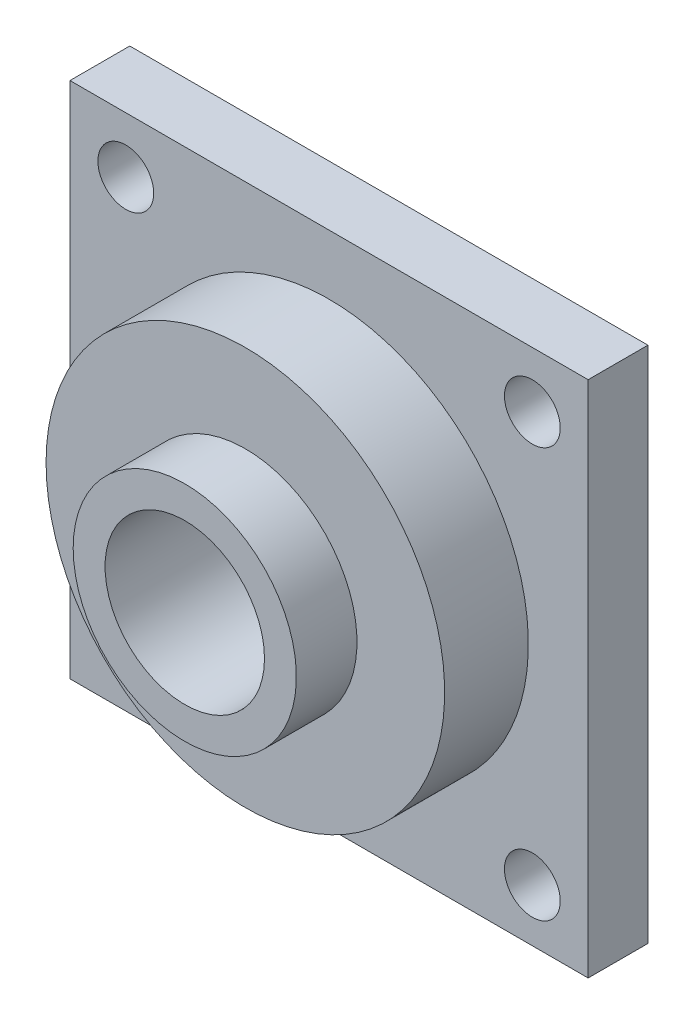
ISO-10303-21;
HEADER;
FILE_DESCRIPTION(('STEP AP214'),'2;1');
FILE_NAME('part.step','',(''),(''),'','','');
FILE_SCHEMA(('AUTOMOTIVE_DESIGN { 1 0 10303 214 1 1 1 1 }'));
ENDSEC;
DATA;
#1=APPLICATION_CONTEXT('core data for automotive mechanical design processes');
#2=APPLICATION_PROTOCOL_DEFINITION('international standard','automotive_design',2000,#1);
#3=PRODUCT_CONTEXT('',#1,'mechanical');
#4=PRODUCT('Part','Part','',(#3));
#5=PRODUCT_RELATED_PRODUCT_CATEGORY('part','',(#4));
#6=PRODUCT_DEFINITION_FORMATION('','',#4);
#7=PRODUCT_DEFINITION_CONTEXT('part definition',#1,'design');
#8=PRODUCT_DEFINITION('design','',#6,#7);
#9=PRODUCT_DEFINITION_SHAPE('','',#8);
#10=(LENGTH_UNIT() NAMED_UNIT(*) SI_UNIT(.MILLI.,.METRE.));
#11=(NAMED_UNIT(*) PLANE_ANGLE_UNIT() SI_UNIT($,.RADIAN.));
#12=(NAMED_UNIT(*) SI_UNIT($,.STERADIAN.) SOLID_ANGLE_UNIT());
#13=UNCERTAINTY_MEASURE_WITH_UNIT(LENGTH_MEASURE(1.E-05),#10,'distance_accuracy_value','');
#14=(GEOMETRIC_REPRESENTATION_CONTEXT(3) GLOBAL_UNCERTAINTY_ASSIGNED_CONTEXT((#13)) GLOBAL_UNIT_ASSIGNED_CONTEXT((#10,
#11,#12)) REPRESENTATION_CONTEXT('',''));
#15=CARTESIAN_POINT('',(0.,0.,0.));
#16=DIRECTION('',(0.,0.,1.));
#17=DIRECTION('',(1.,0.,0.));
#18=AXIS2_PLACEMENT_3D('',#15,#16,#17);
#19=CARTESIAN_POINT('',(0.,130.,15.));
#20=DIRECTION('',(1.,0.,0.));
#21=DIRECTION('',(0.,0.,-1.));
#22=AXIS2_PLACEMENT_3D('',#19,#20,#21);
#23=PLANE('',#22);
#24=DIRECTION('',(0.,-1.,0.));
#25=VECTOR('',#24,1.);
#26=CARTESIAN_POINT('',(0.,130.,0.));
#27=LINE('',#26,#25);
#28=CARTESIAN_POINT('',(0.,130.,0.));
#29=VERTEX_POINT('',#28);
#30=CARTESIAN_POINT('',(0.,0.,0.));
#31=VERTEX_POINT('',#30);
#32=EDGE_CURVE('E115',#29,#31,#27,.T.);
#33=ORIENTED_EDGE('',*,*,#32,.T.);
#34=DIRECTION('',(0.,0.,-1.));
#35=VECTOR('',#34,1.);
#36=CARTESIAN_POINT('',(0.,0.,15.));
#37=LINE('',#36,#35);
#38=CARTESIAN_POINT('',(0.,0.,15.));
#39=VERTEX_POINT('',#38);
#40=EDGE_CURVE('E48',#39,#31,#37,.T.);
#41=ORIENTED_EDGE('',*,*,#40,.F.);
#42=DIRECTION('',(0.,-1.,0.));
#43=VECTOR('',#42,1.);
#44=CARTESIAN_POINT('',(0.,130.,15.));
#45=LINE('',#44,#43);
#46=CARTESIAN_POINT('',(0.,130.,15.));
#47=VERTEX_POINT('',#46);
#48=EDGE_CURVE('E97',#47,#39,#45,.T.);
#49=ORIENTED_EDGE('',*,*,#48,.F.);
#50=DIRECTION('',(0.,0.,-1.));
#51=VECTOR('',#50,1.);
#52=CARTESIAN_POINT('',(0.,130.,15.));
#53=LINE('',#52,#51);
#54=EDGE_CURVE('E107',#47,#29,#53,.T.);
#55=ORIENTED_EDGE('',*,*,#54,.T.);
#56=EDGE_LOOP('',(#33,#41,#49,#55));
#57=FACE_BOUND('',#56,.T.);
#58=ADVANCED_FACE('F44',(#57),#23,.F.);
#59=CARTESIAN_POINT('',(0.,0.,15.));
#60=DIRECTION('',(0.,1.,0.));
#61=DIRECTION('',(0.,0.,1.));
#62=AXIS2_PLACEMENT_3D('',#59,#60,#61);
#63=PLANE('',#62);
#64=DIRECTION('',(1.,0.,0.));
#65=VECTOR('',#64,1.);
#66=CARTESIAN_POINT('',(0.,0.,0.));
#67=LINE('',#66,#65);
#68=CARTESIAN_POINT('',(130.,0.,0.));
#69=VERTEX_POINT('',#68);
#70=EDGE_CURVE('E102',#31,#69,#67,.T.);
#71=ORIENTED_EDGE('',*,*,#70,.T.);
#72=DIRECTION('',(0.,0.,-1.));
#73=VECTOR('',#72,1.);
#74=CARTESIAN_POINT('',(130.,0.,15.));
#75=LINE('',#74,#73);
#76=CARTESIAN_POINT('',(130.,0.,15.));
#77=VERTEX_POINT('',#76);
#78=EDGE_CURVE('E105',#77,#69,#75,.T.);
#79=ORIENTED_EDGE('',*,*,#78,.F.);
#80=DIRECTION('',(1.,0.,0.));
#81=VECTOR('',#80,1.);
#82=CARTESIAN_POINT('',(0.,0.,15.));
#83=LINE('',#82,#81);
#84=EDGE_CURVE('E94',#39,#77,#83,.T.);
#85=ORIENTED_EDGE('',*,*,#84,.F.);
#86=ORIENTED_EDGE('',*,*,#40,.T.);
#87=EDGE_LOOP('',(#71,#79,#85,#86));
#88=FACE_BOUND('',#87,.T.);
#89=ADVANCED_FACE('F103',(#88),#63,.F.);
#90=CARTESIAN_POINT('',(130.,0.,15.));
#91=DIRECTION('',(-1.,0.,0.));
#92=DIRECTION('',(0.,0.,1.));
#93=AXIS2_PLACEMENT_3D('',#90,#91,#92);
#94=PLANE('',#93);
#95=DIRECTION('',(0.,1.,0.));
#96=VECTOR('',#95,1.);
#97=CARTESIAN_POINT('',(130.,0.,0.));
#98=LINE('',#97,#96);
#99=CARTESIAN_POINT('',(130.,130.,0.));
#100=VERTEX_POINT('',#99);
#101=EDGE_CURVE('E76',#69,#100,#98,.T.);
#102=ORIENTED_EDGE('',*,*,#101,.T.);
#103=DIRECTION('',(0.,0.,-1.));
#104=VECTOR('',#103,1.);
#105=CARTESIAN_POINT('',(130.,130.,15.));
#106=LINE('',#105,#104);
#107=CARTESIAN_POINT('',(130.,130.,15.));
#108=VERTEX_POINT('',#107);
#109=EDGE_CURVE('E104',#108,#100,#106,.T.);
#110=ORIENTED_EDGE('',*,*,#109,.F.);
#111=DIRECTION('',(0.,1.,0.));
#112=VECTOR('',#111,1.);
#113=CARTESIAN_POINT('',(130.,0.,15.));
#114=LINE('',#113,#112);
#115=EDGE_CURVE('E100',#77,#108,#114,.T.);
#116=ORIENTED_EDGE('',*,*,#115,.F.);
#117=ORIENTED_EDGE('',*,*,#78,.T.);
#118=EDGE_LOOP('',(#102,#110,#116,#117));
#119=FACE_BOUND('',#118,.T.);
#120=ADVANCED_FACE('F106',(#119),#94,.F.);
#121=CARTESIAN_POINT('',(130.,130.,15.));
#122=DIRECTION('',(0.,-1.,0.));
#123=DIRECTION('',(0.,0.,-1.));
#124=AXIS2_PLACEMENT_3D('',#121,#122,#123);
#125=PLANE('',#124);
#126=DIRECTION('',(-1.,0.,0.));
#127=VECTOR('',#126,1.);
#128=CARTESIAN_POINT('',(130.,130.,0.));
#129=LINE('',#128,#127);
#130=EDGE_CURVE('E88',#100,#29,#129,.T.);
#131=ORIENTED_EDGE('',*,*,#130,.T.);
#132=ORIENTED_EDGE('',*,*,#54,.F.);
#133=DIRECTION('',(-1.,0.,0.));
#134=VECTOR('',#133,1.);
#135=CARTESIAN_POINT('',(130.,130.,15.));
#136=LINE('',#135,#134);
#137=EDGE_CURVE('E63',#108,#47,#136,.T.);
#138=ORIENTED_EDGE('',*,*,#137,.F.);
#139=ORIENTED_EDGE('',*,*,#109,.T.);
#140=EDGE_LOOP('',(#131,#132,#138,#139));
#141=FACE_BOUND('',#140,.T.);
#142=ADVANCED_FACE('F116',(#141),#125,.F.);
#143=CARTESIAN_POINT('',(0.,0.,15.));
#144=DIRECTION('',(0.,0.,1.));
#145=DIRECTION('',(1.,0.,0.));
#146=AXIS2_PLACEMENT_3D('',#143,#144,#145);
#147=PLANE('',#146);
#148=CARTESIAN_POINT('',(116.,13.1965117975312,15.));
#149=DIRECTION('',(0.,0.,1.));
#150=DIRECTION('',(1.,0.,0.));
#151=AXIS2_PLACEMENT_3D('',#148,#149,#150);
#152=CIRCLE('',#151,7.);
#153=CARTESIAN_POINT('',(123.,13.1965117975312,15.));
#154=VERTEX_POINT('',#153);
#155=EDGE_CURVE('E148',#154,#154,#152,.T.);
#156=ORIENTED_EDGE('',*,*,#155,.F.);
#157=EDGE_LOOP('',(#156));
#158=FACE_BOUND('',#157,.T.);
#159=CARTESIAN_POINT('',(14.,14.,15.));
#160=DIRECTION('',(0.,0.,1.));
#161=DIRECTION('',(1.,0.,0.));
#162=AXIS2_PLACEMENT_3D('',#159,#160,#161);
#163=CIRCLE('',#162,7.);
#164=CARTESIAN_POINT('',(21.,14.,15.));
#165=VERTEX_POINT('',#164);
#166=EDGE_CURVE('E155',#165,#165,#163,.T.);
#167=ORIENTED_EDGE('',*,*,#166,.F.);
#168=EDGE_LOOP('',(#167));
#169=FACE_BOUND('',#168,.T.);
#170=CARTESIAN_POINT('',(14.,116.,15.));
#171=DIRECTION('',(0.,0.,1.));
#172=DIRECTION('',(1.,0.,0.));
#173=AXIS2_PLACEMENT_3D('',#170,#171,#172);
#174=CIRCLE('',#173,7.00000000000001);
#175=CARTESIAN_POINT('',(21.,116.,15.));
#176=VERTEX_POINT('',#175);
#177=EDGE_CURVE('E158',#176,#176,#174,.T.);
#178=ORIENTED_EDGE('',*,*,#177,.F.);
#179=EDGE_LOOP('',(#178));
#180=FACE_BOUND('',#179,.T.);
#181=CARTESIAN_POINT('',(116.,116.,15.));
#182=DIRECTION('',(0.,0.,1.));
#183=DIRECTION('',(1.,0.,0.));
#184=AXIS2_PLACEMENT_3D('',#181,#182,#183);
#185=CIRCLE('',#184,7.);
#186=CARTESIAN_POINT('',(123.,116.,15.));
#187=VERTEX_POINT('',#186);
#188=EDGE_CURVE('E137',#187,#187,#185,.T.);
#189=ORIENTED_EDGE('',*,*,#188,.F.);
#190=EDGE_LOOP('',(#189));
#191=FACE_BOUND('',#190,.T.);
#192=CARTESIAN_POINT('',(65.,65.,15.));
#193=DIRECTION('',(0.,0.,1.));
#194=DIRECTION('',(1.,0.,0.));
#195=AXIS2_PLACEMENT_3D('',#192,#193,#194);
#196=CIRCLE('',#195,50.);
#197=CARTESIAN_POINT('',(15.,65.,15.));
#198=VERTEX_POINT('',#197);
#199=EDGE_CURVE('E53',#198,#198,#196,.T.);
#200=ORIENTED_EDGE('',*,*,#199,.F.);
#201=EDGE_LOOP('',(#200));
#202=FACE_BOUND('',#201,.T.);
#203=ORIENTED_EDGE('',*,*,#48,.T.);
#204=ORIENTED_EDGE('',*,*,#84,.T.);
#205=ORIENTED_EDGE('',*,*,#115,.T.);
#206=ORIENTED_EDGE('',*,*,#137,.T.);
#207=EDGE_LOOP('',(#203,#204,#205,#206));
#208=FACE_BOUND('',#207,.T.);
#209=ADVANCED_FACE('F92',(#158,#169,#180,#191,#202,#208),#147,.T.);
#210=CARTESIAN_POINT('',(0.,0.,0.));
#211=DIRECTION('',(0.,0.,1.));
#212=DIRECTION('',(1.,0.,0.));
#213=AXIS2_PLACEMENT_3D('',#210,#211,#212);
#214=PLANE('',#213);
#215=CARTESIAN_POINT('',(116.,13.1965117975312,0.));
#216=DIRECTION('',(0.,0.,1.));
#217=DIRECTION('',(1.,0.,0.));
#218=AXIS2_PLACEMENT_3D('',#215,#216,#217);
#219=CIRCLE('',#218,7.);
#220=CARTESIAN_POINT('',(123.,13.1965117975312,0.));
#221=VERTEX_POINT('',#220);
#222=EDGE_CURVE('E149',#221,#221,#219,.T.);
#223=ORIENTED_EDGE('',*,*,#222,.T.);
#224=EDGE_LOOP('',(#223));
#225=FACE_BOUND('',#224,.T.);
#226=CARTESIAN_POINT('',(14.,14.,0.));
#227=DIRECTION('',(0.,0.,1.));
#228=DIRECTION('',(1.,0.,0.));
#229=AXIS2_PLACEMENT_3D('',#226,#227,#228);
#230=CIRCLE('',#229,7.);
#231=CARTESIAN_POINT('',(21.,14.,0.));
#232=VERTEX_POINT('',#231);
#233=EDGE_CURVE('E154',#232,#232,#230,.T.);
#234=ORIENTED_EDGE('',*,*,#233,.T.);
#235=EDGE_LOOP('',(#234));
#236=FACE_BOUND('',#235,.T.);
#237=CARTESIAN_POINT('',(14.,116.,0.));
#238=DIRECTION('',(0.,0.,1.));
#239=DIRECTION('',(1.,0.,0.));
#240=AXIS2_PLACEMENT_3D('',#237,#238,#239);
#241=CIRCLE('',#240,7.00000000000001);
#242=CARTESIAN_POINT('',(21.,116.,0.));
#243=VERTEX_POINT('',#242);
#244=EDGE_CURVE('E141',#243,#243,#241,.T.);
#245=ORIENTED_EDGE('',*,*,#244,.T.);
#246=EDGE_LOOP('',(#245));
#247=FACE_BOUND('',#246,.T.);
#248=CARTESIAN_POINT('',(116.,116.,0.));
#249=DIRECTION('',(0.,0.,1.));
#250=DIRECTION('',(1.,0.,0.));
#251=AXIS2_PLACEMENT_3D('',#248,#249,#250);
#252=CIRCLE('',#251,7.);
#253=CARTESIAN_POINT('',(123.,116.,0.));
#254=VERTEX_POINT('',#253);
#255=EDGE_CURVE('E136',#254,#254,#252,.T.);
#256=ORIENTED_EDGE('',*,*,#255,.T.);
#257=EDGE_LOOP('',(#256));
#258=FACE_BOUND('',#257,.T.);
#259=CARTESIAN_POINT('',(65.,65.,0.));
#260=DIRECTION('',(0.,0.,1.));
#261=DIRECTION('',(1.,0.,0.));
#262=AXIS2_PLACEMENT_3D('',#259,#260,#261);
#263=CIRCLE('',#262,20.);
#264=CARTESIAN_POINT('',(85.,65.,0.));
#265=VERTEX_POINT('',#264);
#266=EDGE_CURVE('E133',#265,#265,#263,.T.);
#267=ORIENTED_EDGE('',*,*,#266,.T.);
#268=EDGE_LOOP('',(#267));
#269=FACE_BOUND('',#268,.T.);
#270=ORIENTED_EDGE('',*,*,#32,.F.);
#271=ORIENTED_EDGE('',*,*,#130,.F.);
#272=ORIENTED_EDGE('',*,*,#101,.F.);
#273=ORIENTED_EDGE('',*,*,#70,.F.);
#274=EDGE_LOOP('',(#270,#271,#272,#273));
#275=FACE_BOUND('',#274,.T.);
#276=ADVANCED_FACE('F125',(#225,#236,#247,#258,#269,#275),#214,.F.);
#277=CARTESIAN_POINT('',(65.,65.,36.));
#278=DIRECTION('',(0.,0.,-1.));
#279=DIRECTION('',(-1.,0.,0.));
#280=AXIS2_PLACEMENT_3D('',#277,#278,#279);
#281=CYLINDRICAL_SURFACE('',#280,50.);
#282=CARTESIAN_POINT('',(65.,65.,36.));
#283=DIRECTION('',(0.,0.,1.));
#284=DIRECTION('',(1.,0.,0.));
#285=AXIS2_PLACEMENT_3D('',#282,#283,#284);
#286=CIRCLE('',#285,50.);
#287=CARTESIAN_POINT('',(15.,65.,36.));
#288=VERTEX_POINT('',#287);
#289=EDGE_CURVE('E113',#288,#288,#286,.T.);
#290=CARTESIAN_POINT('',(15.,65.,36.));
#291=CARTESIAN_POINT('',(15.,65.,35.78125));
#292=CARTESIAN_POINT('',(15.,65.,35.5625));
#293=CARTESIAN_POINT('',(15.,65.,35.125));
#294=CARTESIAN_POINT('',(15.,65.,34.90625));
#295=CARTESIAN_POINT('',(15.,65.,34.46875));
#296=CARTESIAN_POINT('',(15.,65.,34.25));
#297=CARTESIAN_POINT('',(15.,65.,33.8125));
#298=CARTESIAN_POINT('',(15.,65.,33.59375));
#299=CARTESIAN_POINT('',(15.,65.,33.15625));
#300=CARTESIAN_POINT('',(15.,65.,32.9375));
#301=CARTESIAN_POINT('',(15.,65.,32.5));
#302=CARTESIAN_POINT('',(15.,65.,32.28125));
#303=CARTESIAN_POINT('',(15.,65.,31.84375));
#304=CARTESIAN_POINT('',(15.,65.,31.625));
#305=CARTESIAN_POINT('',(15.,65.,31.1875));
#306=CARTESIAN_POINT('',(15.,65.,30.96875));
#307=CARTESIAN_POINT('',(15.,65.,30.53125));
#308=CARTESIAN_POINT('',(15.,65.,30.3125));
#309=CARTESIAN_POINT('',(15.,65.,29.875));
#310=CARTESIAN_POINT('',(15.,65.,29.65625));
#311=CARTESIAN_POINT('',(15.,65.,29.21875));
#312=CARTESIAN_POINT('',(15.,65.,29.));
#313=CARTESIAN_POINT('',(15.,65.,28.5625));
#314=CARTESIAN_POINT('',(15.,65.,28.34375));
#315=CARTESIAN_POINT('',(15.,65.,27.90625));
#316=CARTESIAN_POINT('',(15.,65.,27.6875));
#317=CARTESIAN_POINT('',(15.,65.,27.25));
#318=CARTESIAN_POINT('',(15.,65.,27.03125));
#319=CARTESIAN_POINT('',(15.,65.,26.59375));
#320=CARTESIAN_POINT('',(15.,65.,26.375));
#321=CARTESIAN_POINT('',(15.,65.,25.9375));
#322=CARTESIAN_POINT('',(15.,65.,25.71875));
#323=CARTESIAN_POINT('',(15.,65.,25.28125));
#324=CARTESIAN_POINT('',(15.,65.,25.0625));
#325=CARTESIAN_POINT('',(15.,65.,24.625));
#326=CARTESIAN_POINT('',(15.,65.,24.40625));
#327=CARTESIAN_POINT('',(15.,65.,23.96875));
#328=CARTESIAN_POINT('',(15.,65.,23.75));
#329=CARTESIAN_POINT('',(15.,65.,23.3125));
#330=CARTESIAN_POINT('',(15.,65.,23.09375));
#331=CARTESIAN_POINT('',(15.,65.,22.65625));
#332=CARTESIAN_POINT('',(15.,65.,22.4375));
#333=CARTESIAN_POINT('',(15.,65.,22.));
#334=CARTESIAN_POINT('',(15.,65.,21.78125));
#335=CARTESIAN_POINT('',(15.,65.,21.34375));
#336=CARTESIAN_POINT('',(15.,65.,21.125));
#337=CARTESIAN_POINT('',(15.,65.,20.6875));
#338=CARTESIAN_POINT('',(15.,65.,20.46875));
#339=CARTESIAN_POINT('',(15.,65.,20.03125));
#340=CARTESIAN_POINT('',(15.,65.,19.8125));
#341=CARTESIAN_POINT('',(15.,65.,19.375));
#342=CARTESIAN_POINT('',(15.,65.,19.15625));
#343=CARTESIAN_POINT('',(15.,65.,18.71875));
#344=CARTESIAN_POINT('',(15.,65.,18.5));
#345=CARTESIAN_POINT('',(15.,65.,18.0625));
#346=CARTESIAN_POINT('',(15.,65.,17.84375));
#347=CARTESIAN_POINT('',(15.,65.,17.40625));
#348=CARTESIAN_POINT('',(15.,65.,17.1875));
#349=CARTESIAN_POINT('',(15.,65.,16.75));
#350=CARTESIAN_POINT('',(15.,65.,16.53125));
#351=CARTESIAN_POINT('',(15.,65.,16.09375));
#352=CARTESIAN_POINT('',(15.,65.,15.875));
#353=CARTESIAN_POINT('',(15.,65.,15.4375));
#354=CARTESIAN_POINT('',(15.,65.,15.21875));
#355=CARTESIAN_POINT('',(15.,65.,15.));
#356=B_SPLINE_CURVE_WITH_KNOTS('',3,(#290,#291,#292,#293,#294,#295,#296,#297,#298,#299,#300,
#301,#302,#303,#304,#305,#306,#307,#308,#309,#310,#311,#312,#313,#314,#315,#316,#317,#318,#319,
#320,#321,#322,#323,#324,#325,#326,#327,#328,#329,#330,#331,#332,#333,#334,#335,#336,#337,#338,
#339,#340,#341,#342,#343,#344,#345,#346,#347,#348,#349,#350,#351,#352,#353,#354,#355),
.UNSPECIFIED.,.F.,.F.,(4,2,2,2,2,2,2,2,2,2,2,2,2,2,2,2,2,2,2,2,2,2,2,2,2,2,2,2,2,2,2,2,4),(0.,
0.656250000000004,1.3125,1.96875000000001,2.625,3.28125000000001,3.9375,4.59375000000001,5.25,
5.90625000000001,6.56250000000001,7.21875000000001,7.87500000000001,8.53125,9.18750000000001,
9.84375000000001,10.5,11.15625,11.8125,12.46875,13.125,13.78125,14.4375,15.09375,15.75,16.40625,
17.0625,17.71875,18.375,19.03125,19.6875,20.34375,21.),.UNSPECIFIED.);
#357=EDGE_CURVE('BSEAM185',#288,#198,#356,.T.);
#358=ORIENTED_EDGE('',*,*,#289,.F.);
#359=ORIENTED_EDGE('',*,*,#199,.T.);
#360=ORIENTED_EDGE('',*,*,#357,.T.);
#361=ORIENTED_EDGE('',*,*,#357,.F.);
#362=EDGE_LOOP('',(#358,#360,#359,#361));
#363=FACE_BOUND('',#362,.T.);
#364=ADVANCED_FACE('F185',(#363),#281,.T.);
#365=CARTESIAN_POINT('',(65.,65.,36.));
#366=DIRECTION('',(0.,0.,1.));
#367=DIRECTION('',(1.,0.,0.));
#368=AXIS2_PLACEMENT_3D('',#365,#366,#367);
#369=PLANE('',#368);
#370=CARTESIAN_POINT('',(65.,65.,36.));
#371=DIRECTION('',(0.,0.,1.));
#372=DIRECTION('',(1.,0.,0.));
#373=AXIS2_PLACEMENT_3D('',#370,#371,#372);
#374=CIRCLE('',#373,28.);
#375=CARTESIAN_POINT('',(37.,65.,36.));
#376=VERTEX_POINT('',#375);
#377=EDGE_CURVE('E11',#376,#376,#374,.T.);
#378=ORIENTED_EDGE('',*,*,#377,.F.);
#379=EDGE_LOOP('',(#378));
#380=FACE_BOUND('',#379,.T.);
#381=ORIENTED_EDGE('',*,*,#289,.T.);
#382=EDGE_LOOP('',(#381));
#383=FACE_BOUND('',#382,.T.);
#384=ADVANCED_FACE('F184',(#380,#383),#369,.T.);
#385=CARTESIAN_POINT('',(65.,65.,51.2));
#386=DIRECTION('',(0.,0.,-1.));
#387=DIRECTION('',(-1.,0.,0.));
#388=AXIS2_PLACEMENT_3D('',#385,#386,#387);
#389=CYLINDRICAL_SURFACE('',#388,28.);
#390=CARTESIAN_POINT('',(65.,65.,51.2));
#391=DIRECTION('',(0.,0.,1.));
#392=DIRECTION('',(1.,0.,0.));
#393=AXIS2_PLACEMENT_3D('',#390,#391,#392);
#394=CIRCLE('',#393,28.);
#395=CARTESIAN_POINT('',(37.,65.,51.2));
#396=VERTEX_POINT('',#395);
#397=EDGE_CURVE('E129',#396,#396,#394,.T.);
#398=CARTESIAN_POINT('',(37.,65.,51.2));
#399=CARTESIAN_POINT('',(37.,65.,51.0416666666667));
#400=CARTESIAN_POINT('',(37.,65.,50.8833333333333));
#401=CARTESIAN_POINT('',(37.,65.,50.5666666666667));
#402=CARTESIAN_POINT('',(37.,65.,50.4083333333333));
#403=CARTESIAN_POINT('',(37.,65.,50.0916666666667));
#404=CARTESIAN_POINT('',(37.,65.,49.9333333333333));
#405=CARTESIAN_POINT('',(37.,65.,49.6166666666667));
#406=CARTESIAN_POINT('',(37.,65.,49.4583333333333));
#407=CARTESIAN_POINT('',(37.,65.,49.1416666666667));
#408=CARTESIAN_POINT('',(37.,65.,48.9833333333333));
#409=CARTESIAN_POINT('',(37.,65.,48.6666666666667));
#410=CARTESIAN_POINT('',(37.,65.,48.5083333333333));
#411=CARTESIAN_POINT('',(37.,65.,48.1916666666667));
#412=CARTESIAN_POINT('',(37.,65.,48.0333333333333));
#413=CARTESIAN_POINT('',(37.,65.,47.7166666666667));
#414=CARTESIAN_POINT('',(37.,65.,47.5583333333333));
#415=CARTESIAN_POINT('',(37.,65.,47.2416666666667));
#416=CARTESIAN_POINT('',(37.,65.,47.0833333333333));
#417=CARTESIAN_POINT('',(37.,65.,46.7666666666667));
#418=CARTESIAN_POINT('',(37.,65.,46.6083333333333));
#419=CARTESIAN_POINT('',(37.,65.,46.2916666666667));
#420=CARTESIAN_POINT('',(37.,65.,46.1333333333333));
#421=CARTESIAN_POINT('',(37.,65.,45.8166666666667));
#422=CARTESIAN_POINT('',(37.,65.,45.6583333333333));
#423=CARTESIAN_POINT('',(37.,65.,45.3416666666667));
#424=CARTESIAN_POINT('',(37.,65.,45.1833333333333));
#425=CARTESIAN_POINT('',(37.,65.,44.8666666666667));
#426=CARTESIAN_POINT('',(37.,65.,44.7083333333333));
#427=CARTESIAN_POINT('',(37.,65.,44.3916666666667));
#428=CARTESIAN_POINT('',(37.,65.,44.2333333333333));
#429=CARTESIAN_POINT('',(37.,65.,43.9166666666667));
#430=CARTESIAN_POINT('',(37.,65.,43.7583333333333));
#431=CARTESIAN_POINT('',(37.,65.,43.4416666666667));
#432=CARTESIAN_POINT('',(37.,65.,43.2833333333333));
#433=CARTESIAN_POINT('',(37.,65.,42.9666666666667));
#434=CARTESIAN_POINT('',(37.,65.,42.8083333333333));
#435=CARTESIAN_POINT('',(37.,65.,42.4916666666667));
#436=CARTESIAN_POINT('',(37.,65.,42.3333333333333));
#437=CARTESIAN_POINT('',(37.,65.,42.0166666666667));
#438=CARTESIAN_POINT('',(37.,65.,41.8583333333333));
#439=CARTESIAN_POINT('',(37.,65.,41.5416666666667));
#440=CARTESIAN_POINT('',(37.,65.,41.3833333333333));
#441=CARTESIAN_POINT('',(37.,65.,41.0666666666667));
#442=CARTESIAN_POINT('',(37.,65.,40.9083333333333));
#443=CARTESIAN_POINT('',(37.,65.,40.5916666666667));
#444=CARTESIAN_POINT('',(37.,65.,40.4333333333333));
#445=CARTESIAN_POINT('',(37.,65.,40.1166666666667));
#446=CARTESIAN_POINT('',(37.,65.,39.9583333333333));
#447=CARTESIAN_POINT('',(37.,65.,39.6416666666667));
#448=CARTESIAN_POINT('',(37.,65.,39.4833333333333));
#449=CARTESIAN_POINT('',(37.,65.,39.1666666666667));
#450=CARTESIAN_POINT('',(37.,65.,39.0083333333333));
#451=CARTESIAN_POINT('',(37.,65.,38.6916666666667));
#452=CARTESIAN_POINT('',(37.,65.,38.5333333333333));
#453=CARTESIAN_POINT('',(37.,65.,38.2166666666667));
#454=CARTESIAN_POINT('',(37.,65.,38.0583333333333));
#455=CARTESIAN_POINT('',(37.,65.,37.7416666666667));
#456=CARTESIAN_POINT('',(37.,65.,37.5833333333333));
#457=CARTESIAN_POINT('',(37.,65.,37.2666666666667));
#458=CARTESIAN_POINT('',(37.,65.,37.1083333333333));
#459=CARTESIAN_POINT('',(37.,65.,36.7916666666667));
#460=CARTESIAN_POINT('',(37.,65.,36.6333333333333));
#461=CARTESIAN_POINT('',(37.,65.,36.3166666666667));
#462=CARTESIAN_POINT('',(37.,65.,36.1583333333333));
#463=CARTESIAN_POINT('',(37.,65.,36.));
#464=B_SPLINE_CURVE_WITH_KNOTS('',3,(#398,#399,#400,#401,#402,#403,#404,#405,#406,#407,#408,
#409,#410,#411,#412,#413,#414,#415,#416,#417,#418,#419,#420,#421,#422,#423,#424,#425,#426,#427,
#428,#429,#430,#431,#432,#433,#434,#435,#436,#437,#438,#439,#440,#441,#442,#443,#444,#445,#446,
#447,#448,#449,#450,#451,#452,#453,#454,#455,#456,#457,#458,#459,#460,#461,#462,#463),
.UNSPECIFIED.,.F.,.F.,(4,2,2,2,2,2,2,2,2,2,2,2,2,2,2,2,2,2,2,2,2,2,2,2,2,2,2,2,2,2,2,2,4),(0.,
0.475000000000003,0.950000000000006,1.425,1.90000000000001,2.375,2.85000000000001,3.325,3.8,
4.275,4.75,5.225,5.7,6.17500000000001,6.65,7.12500000000001,7.6,8.07500000000001,8.55,
9.02500000000001,9.5,9.975,10.45,10.925,11.4,11.875,12.35,12.825,13.3,13.775,14.25,14.725,15.2),.UNSPECIFIED.);
#465=EDGE_CURVE('BSEAM194',#396,#376,#464,.T.);
#466=ORIENTED_EDGE('',*,*,#397,.F.);
#467=ORIENTED_EDGE('',*,*,#377,.T.);
#468=ORIENTED_EDGE('',*,*,#465,.T.);
#469=ORIENTED_EDGE('',*,*,#465,.F.);
#470=EDGE_LOOP('',(#466,#468,#467,#469));
#471=FACE_BOUND('',#470,.T.);
#472=ADVANCED_FACE('F194',(#471),#389,.T.);
#473=CARTESIAN_POINT('',(65.,65.,51.2));
#474=DIRECTION('',(0.,0.,1.));
#475=DIRECTION('',(1.,0.,0.));
#476=AXIS2_PLACEMENT_3D('',#473,#474,#475);
#477=PLANE('',#476);
#478=CARTESIAN_POINT('',(65.,65.,51.2));
#479=DIRECTION('',(0.,0.,1.));
#480=DIRECTION('',(1.,0.,0.));
#481=AXIS2_PLACEMENT_3D('',#478,#479,#480);
#482=CIRCLE('',#481,20.);
#483=CARTESIAN_POINT('',(85.,65.,51.2));
#484=VERTEX_POINT('',#483);
#485=EDGE_CURVE('E134',#484,#484,#482,.T.);
#486=ORIENTED_EDGE('',*,*,#485,.F.);
#487=EDGE_LOOP('',(#486));
#488=FACE_BOUND('',#487,.T.);
#489=ORIENTED_EDGE('',*,*,#397,.T.);
#490=EDGE_LOOP('',(#489));
#491=FACE_BOUND('',#490,.T.);
#492=ADVANCED_FACE('F239',(#488,#491),#477,.T.);
#493=CARTESIAN_POINT('',(65.,65.,0.));
#494=DIRECTION('',(0.,0.,1.));
#495=DIRECTION('',(1.,0.,0.));
#496=AXIS2_PLACEMENT_3D('',#493,#494,#495);
#497=CYLINDRICAL_SURFACE('',#496,20.);
#498=ORIENTED_EDGE('',*,*,#266,.F.);
#499=EDGE_LOOP('',(#498));
#500=FACE_BOUND('',#499,.T.);
#501=ORIENTED_EDGE('',*,*,#485,.T.);
#502=EDGE_LOOP('',(#501));
#503=FACE_BOUND('',#502,.T.);
#504=ADVANCED_FACE('F248',(#500,#503),#497,.F.);
#505=CARTESIAN_POINT('',(116.,116.,0.));
#506=DIRECTION('',(0.,0.,1.));
#507=DIRECTION('',(1.,0.,0.));
#508=AXIS2_PLACEMENT_3D('',#505,#506,#507);
#509=CYLINDRICAL_SURFACE('',#508,7.);
#510=ORIENTED_EDGE('',*,*,#255,.F.);
#511=EDGE_LOOP('',(#510));
#512=FACE_BOUND('',#511,.T.);
#513=ORIENTED_EDGE('',*,*,#188,.T.);
#514=EDGE_LOOP('',(#513));
#515=FACE_BOUND('',#514,.T.);
#516=ADVANCED_FACE('F168',(#512,#515),#509,.F.);
#517=CARTESIAN_POINT('',(14.,116.,0.));
#518=DIRECTION('',(0.,0.,1.));
#519=DIRECTION('',(1.,0.,0.));
#520=AXIS2_PLACEMENT_3D('',#517,#518,#519);
#521=CYLINDRICAL_SURFACE('',#520,7.00000000000001);
#522=ORIENTED_EDGE('',*,*,#244,.F.);
#523=EDGE_LOOP('',(#522));
#524=FACE_BOUND('',#523,.T.);
#525=ORIENTED_EDGE('',*,*,#177,.T.);
#526=EDGE_LOOP('',(#525));
#527=FACE_BOUND('',#526,.T.);
#528=ADVANCED_FACE('F167',(#524,#527),#521,.F.);
#529=CARTESIAN_POINT('',(14.,14.,0.));
#530=DIRECTION('',(0.,0.,1.));
#531=DIRECTION('',(1.,0.,0.));
#532=AXIS2_PLACEMENT_3D('',#529,#530,#531);
#533=CYLINDRICAL_SURFACE('',#532,7.);
#534=ORIENTED_EDGE('',*,*,#233,.F.);
#535=EDGE_LOOP('',(#534));
#536=FACE_BOUND('',#535,.T.);
#537=ORIENTED_EDGE('',*,*,#166,.T.);
#538=EDGE_LOOP('',(#537));
#539=FACE_BOUND('',#538,.T.);
#540=ADVANCED_FACE('F166',(#536,#539),#533,.F.);
#541=CARTESIAN_POINT('',(116.,13.1965117975312,0.));
#542=DIRECTION('',(0.,0.,1.));
#543=DIRECTION('',(1.,0.,0.));
#544=AXIS2_PLACEMENT_3D('',#541,#542,#543);
#545=CYLINDRICAL_SURFACE('',#544,7.);
#546=ORIENTED_EDGE('',*,*,#222,.F.);
#547=EDGE_LOOP('',(#546));
#548=FACE_BOUND('',#547,.T.);
#549=ORIENTED_EDGE('',*,*,#155,.T.);
#550=EDGE_LOOP('',(#549));
#551=FACE_BOUND('',#550,.T.);
#552=ADVANCED_FACE('F284',(#548,#551),#545,.F.);
#553=CLOSED_SHELL('',(#58,#89,#120,#142,#209,#276,#364,#384,#472,#492,#504,#516,#528,#540,#552));
#554=MANIFOLD_SOLID_BREP('B2',#553);
#555=ADVANCED_BREP_SHAPE_REPRESENTATION('',(#18,#554),#14);
#556=SHAPE_DEFINITION_REPRESENTATION(#9,#555);
ENDSEC;
END-ISO-10303-21;
